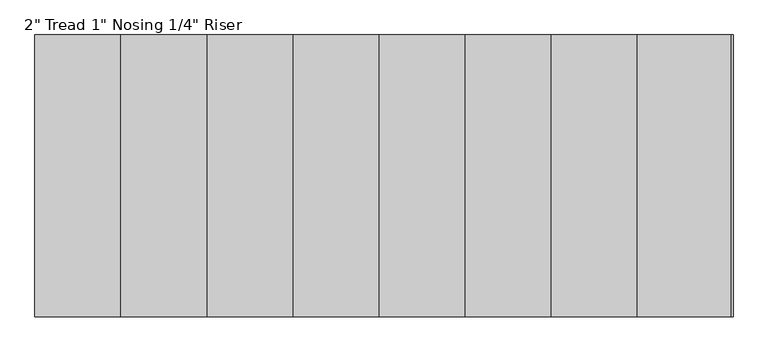
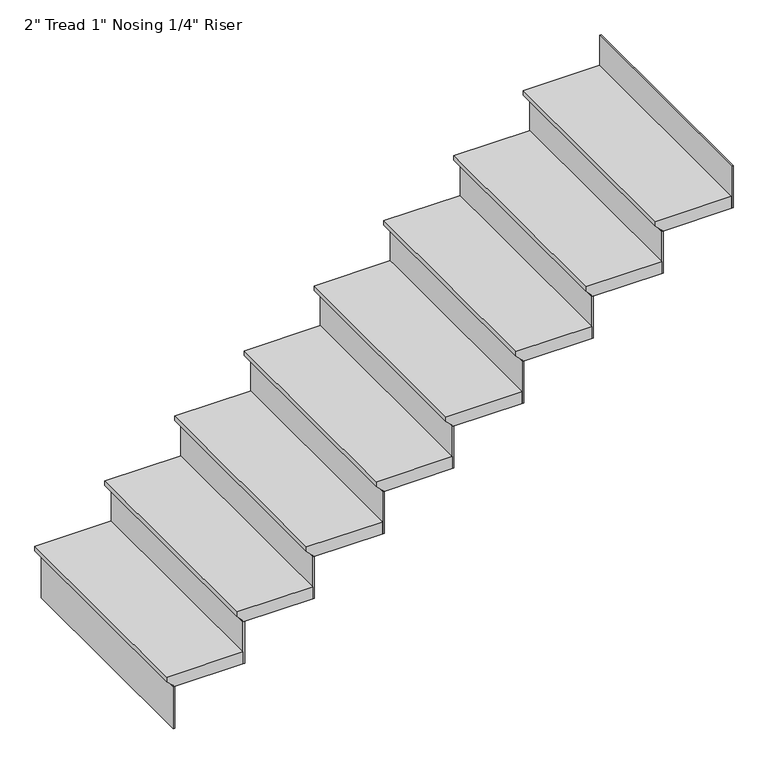
"""IFC4 building model written with IfcOpenShell, lengths in millimetres: stair flight geometry."""

from ifc_helpers import new_model, si_unit, frame, origin, place, context, project, spatial, polyline, outline, extrude, source, transform, mapped, element, save


def stair_flight_79624163(model_context):
    return source(origin(), model_context, "Body", "SweptSolid", [
        extrude(outline(polyline([(8178.8, -5175.7112714), (8178.8, -5480.5112714), (8159.75, -5480.5112714), (8134.35, -5455.1112714), (8128.0, -5455.1112714), (8128.0, -5175.7112714), (8178.8, -5175.7112714)])), frame((0.0, -6800.457676, 0.0), z_axis=(0.0, 1.0, 0.0), x_axis=(0.0, 0.0, 1.0)), (0.0, 0.0, 1.0), 914.4),
        extrude(outline(polyline([(-5448.7612714, -6800.457676), (-5455.1112714, -6800.457676), (-5455.1112714, -5886.057676), (-5448.7612714, -5886.057676), (-5448.7612714, -6800.457676)])), frame((0.0, 0.0, 7950.2), z_axis=(0.0, 0.0, 1.0), x_axis=(1.0, 0.0, 0.0)), (0.0, 0.0, 1.0), 177.8),
        extrude(outline(polyline([(-3213.5612714, -6800.457676), (-3219.9112714, -6800.457676), (-3219.9112714, -5886.057676), (-3213.5612714, -5886.057676), (-3213.5612714, -6800.457676)])), frame((0.0, 0.0, 9372.6), z_axis=(0.0, 0.0, 1.0), x_axis=(1.0, 0.0, 0.0)), (0.0, 0.0, 1.0), 177.8),
        extrude(outline(polyline([(-5169.3612714, -6800.457676), (-5175.7112714, -6800.457676), (-5175.7112714, -5886.057676), (-5169.3612714, -5886.057676), (-5169.3612714, -6800.457676)])), frame((0.0, 0.0, 8128.0), z_axis=(0.0, 0.0, 1.0), x_axis=(1.0, 0.0, 0.0)), (0.0, 0.0, 1.0), 177.8),
        extrude(outline(polyline([(8356.6, -4896.3112714), (8356.6, -5201.1112714), (8337.55, -5201.1112714), (8312.15, -5175.7112714), (8305.8, -5175.7112714), (8305.8, -4896.3112714), (8356.6, -4896.3112714)])), frame((0.0, -6800.457676, 0.0), z_axis=(0.0, 1.0, 0.0), x_axis=(0.0, 0.0, 1.0)), (0.0, 0.0, 1.0), 914.4),
        extrude(outline(polyline([(-4889.9612714, -6800.457676), (-4896.3112714, -6800.457676), (-4896.3112714, -5886.057676), (-4889.9612714, -5886.057676), (-4889.9612714, -6800.457676)])), frame((0.0, 0.0, 8305.8), z_axis=(0.0, 0.0, 1.0), x_axis=(1.0, 0.0, 0.0)), (0.0, 0.0, 1.0), 177.8),
        extrude(outline(polyline([(8534.4, -4616.9112714), (8534.4, -4921.7112714), (8515.35, -4921.7112714), (8489.95, -4896.3112714), (8483.6, -4896.3112714), (8483.6, -4616.9112714), (8534.4, -4616.9112714)])), frame((0.0, -6800.457676, 0.0), z_axis=(0.0, 1.0, 0.0), x_axis=(0.0, 0.0, 1.0)), (0.0, 0.0, 1.0), 914.4),
        extrude(outline(polyline([(-4610.5612714, -6800.457676), (-4616.9112714, -6800.457676), (-4616.9112714, -5886.057676), (-4610.5612714, -5886.057676), (-4610.5612714, -6800.457676)])), frame((0.0, 0.0, 8483.6), z_axis=(0.0, 0.0, 1.0), x_axis=(1.0, 0.0, 0.0)), (0.0, 0.0, 1.0), 177.8),
        extrude(outline(polyline([(8712.2, -4337.5112714), (8712.2, -4642.3112714), (8693.15, -4642.3112714), (8667.75, -4616.9112714), (8661.4, -4616.9112714), (8661.4, -4337.5112714), (8712.2, -4337.5112714)])), frame((0.0, -6800.457676, 0.0), z_axis=(0.0, 1.0, 0.0), x_axis=(0.0, 0.0, 1.0)), (0.0, 0.0, 1.0), 914.4),
        extrude(outline(polyline([(-4331.1612714, -6800.457676), (-4337.5112714, -6800.457676), (-4337.5112714, -5886.057676), (-4331.1612714, -5886.057676), (-4331.1612714, -6800.457676)])), frame((0.0, 0.0, 8661.4), z_axis=(0.0, 0.0, 1.0), x_axis=(1.0, 0.0, 0.0)), (0.0, 0.0, 1.0), 177.8),
        extrude(outline(polyline([(8890.0, -4058.1112714), (8890.0, -4362.9112714), (8870.95, -4362.9112714), (8845.55, -4337.5112714), (8839.2, -4337.5112714), (8839.2, -4058.1112714), (8890.0, -4058.1112714)])), frame((0.0, -6800.457676, 0.0), z_axis=(0.0, 1.0, 0.0), x_axis=(0.0, 0.0, 1.0)), (0.0, 0.0, 1.0), 914.4),
        extrude(outline(polyline([(-4051.7612714, -6800.457676), (-4058.1112714, -6800.457676), (-4058.1112714, -5886.057676), (-4051.7612714, -5886.057676), (-4051.7612714, -6800.457676)])), frame((0.0, 0.0, 8839.2), z_axis=(0.0, 0.0, 1.0), x_axis=(1.0, 0.0, 0.0)), (0.0, 0.0, 1.0), 177.8),
        extrude(outline(polyline([(9067.8, -3778.7112714), (9067.8, -4083.5112714), (9048.75, -4083.5112714), (9023.35, -4058.1112714), (9017.0, -4058.1112714), (9017.0, -3778.7112714), (9067.8, -3778.7112714)])), frame((0.0, -6800.457676, 0.0), z_axis=(0.0, 1.0, 0.0), x_axis=(0.0, 0.0, 1.0)), (0.0, 0.0, 1.0), 914.4),
        extrude(outline(polyline([(-3772.3612714, -6800.457676), (-3778.7112714, -6800.457676), (-3778.7112714, -5886.057676), (-3772.3612714, -5886.057676), (-3772.3612714, -6800.457676)])), frame((0.0, 0.0, 9017.0), z_axis=(0.0, 0.0, 1.0), x_axis=(1.0, 0.0, 0.0)), (0.0, 0.0, 1.0), 177.8),
        extrude(outline(polyline([(9245.6, -3499.3112714), (9245.6, -3804.1112714), (9226.55, -3804.1112714), (9201.15, -3778.7112714), (9194.8, -3778.7112714), (9194.8, -3499.3112714), (9245.6, -3499.3112714)])), frame((0.0, -6800.457676, 0.0), z_axis=(0.0, 1.0, 0.0), x_axis=(0.0, 0.0, 1.0)), (0.0, 0.0, 1.0), 914.4),
        extrude(outline(polyline([(-3492.9612714, -6800.457676), (-3499.3112714, -6800.457676), (-3499.3112714, -5886.057676), (-3492.9612714, -5886.057676), (-3492.9612714, -6800.457676)])), frame((0.0, 0.0, 9194.8), z_axis=(0.0, 0.0, 1.0), x_axis=(1.0, 0.0, 0.0)), (0.0, 0.0, 1.0), 177.8),
        extrude(outline(polyline([(9423.4, -3219.9112714), (9423.4, -3524.7112714), (9404.35, -3524.7112714), (9378.95, -3499.3112714), (9372.6, -3499.3112714), (9372.6, -3219.9112714), (9423.4, -3219.9112714)])), frame((0.0, -6800.457676, 0.0), z_axis=(0.0, 1.0, 0.0), x_axis=(0.0, 0.0, 1.0)), (0.0, 0.0, 1.0), 914.4),
    ])


if __name__ == "__main__":
    model = new_model("IFC4")
    model_context = context("Model", 3, world=origin())
    ifc_project = project(units=[si_unit("LENGTHUNIT", "METRE", prefix="MILLI")], contexts=[model_context])
    site = spatial("IfcSite", under=ifc_project)
    building = spatial("IfcBuilding", under=site)
    placement = place(None, origin())
    stair_flight_shape = stair_flight_79624163(model_context)
    element("IfcStairFlight", 1, ObjectType="2\" Tread 1\" Nosing 1/4\" Riser", at=placement, inside=building, context=model_context, shape_type="MappedRepresentation", body=[
        mapped(stair_flight_shape, transform((0.0, 0.0, 0.0), x_axis=(1.0, 0.0, 0.0), y_axis=(0.0, 1.0, 0.0), z_axis=(0.0, 0.0, 1.0))),
    ])
    save(model, "model.ifc")
